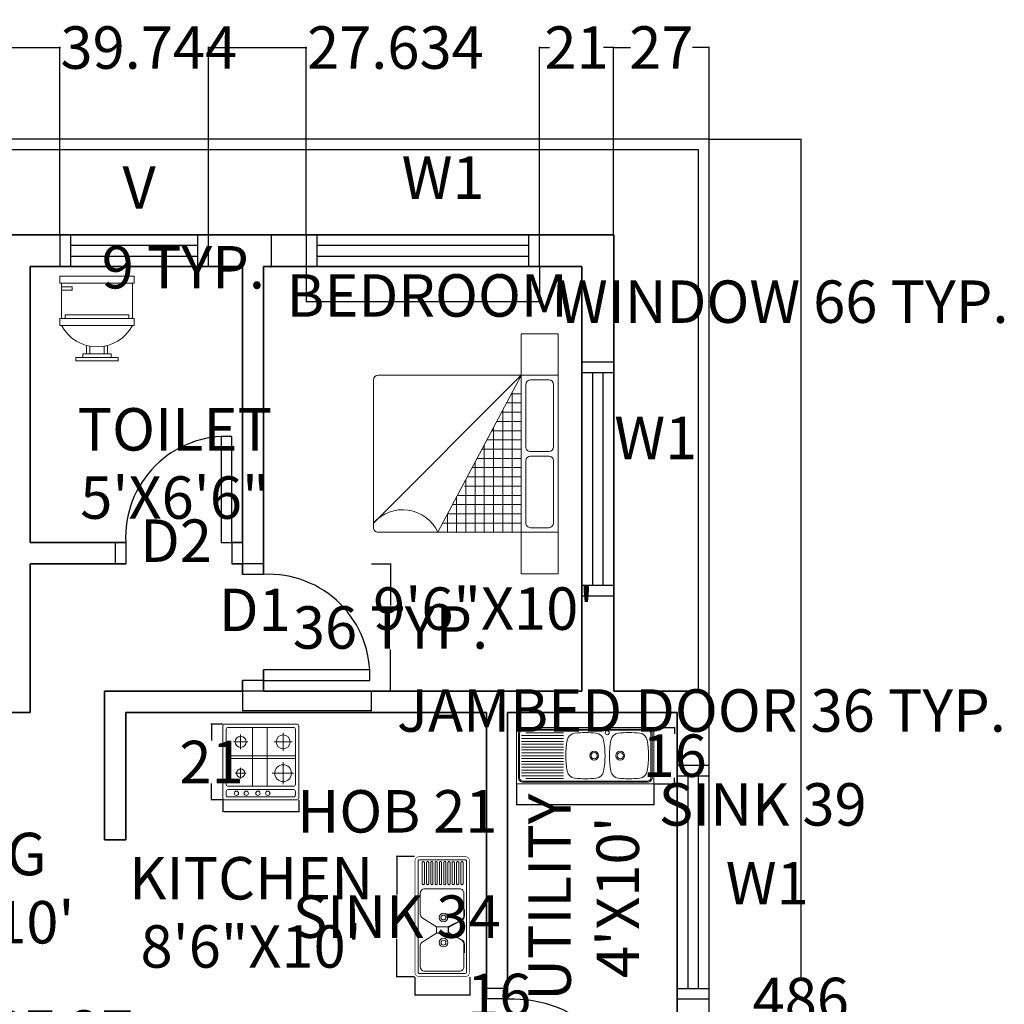
# Model space of a CAD drawing. Units: inches. Extents: x 774 to 1314, y 374 to 930.
# Tile 5 of 5: x 1035 to 1314, y 652 to 930. Entities that reach past the tile are written whole.
import ezdxf
from ezdxf.enums import TextEntityAlignment as Align

# ---------------------------------------------------------------- set-up
doc = ezdxf.new("R2010")
doc.units = ezdxf.units.IN
doc.header["$MEASUREMENT"] = 0
for name, color, linetype, lineweight in [('A-ANNO-DIMS', 2, 'Continuous', 18), ('A-ANNO-TEXT', 2, 'Continuous', 18), ('A-AREA-IDEN', 2, 'Continuous', 18), ('A-DOOR', 6, 'Continuous', 25), ('A-EQPM', 9, 'Continuous', 18), ('A-FLOR-FIXT', 9, 'Continuous', 18), ('A-FURN', 8, 'Continuous', 18), ('A-GLAZ', 4, 'Continuous', 18), ('A-WALL', 1, 'Continuous', 35), ('C-PROP', 3, 'Continuous', 25)]:
    doc.layers.add(name, color=color, linetype=linetype, lineweight=lineweight)
doc.layers.add('Layer4', color=4, linetype='Continuous')
doc.styles.get("Standard").update_dxf_attribs({"font": 'arial.ttf'})
doc.dimstyles.get("Standard").update_dxf_attribs({"dimtxt": 12, "dimasz": 0.18, "dimexe": 0.18, "dimexo": 0.0625, "dimgap": 0.09, "dimtad": 0, "dimtih": 1, "dimtoh": 1, "dimdec": 0, "dimzin": 0, "dimdsep": 46, "dimlunit": 4, "dimtxsty": 'Standard', "dimcen": 0.09, "dimadec": 0, "dimazin": 0, "dimtfac": 1, "dimtdec": 0, "dimtofl": 0, "dimtmove": 0, "dimatfit": 3, "dimfxl": 1, "dimtolj": 1, "dimtzin": 0, "dimarcsym": 0})

# ---------------------------------------------------------------- blocks, each defined once
blk = doc.blocks.new('ty')
at = {"layer": 'Layer4'}
for p, q in [((9, 42), (0, 42)), ((9, 39), (0, 39)), ((0, 39), (0, 3)), ((3, 39), (3, 3)), ((6, 3), (6, 39)), ((9, 3), (9, 39)), ((0, 3), (9, 3)), ((0, 0), (9, 0))]:
    blk.add_line(p, q, dxfattribs=at)
blk = doc.blocks.new('tr')
at = {"layer": 'Layer4'}
for p, q in [((9, 66), (0, 66)), ((9, 63), (0, 63)), ((0, 63), (0, 3)), ((3, 63), (3, 3)), ((6, 3), (6, 63)), ((9, 3), (9, 63)), ((0, 3), (9, 3)), ((0, 0), (9, 0))]:
    blk.add_line(p, q, dxfattribs=at)
blk = doc.blocks.new('A$C4CBC1980')
for p, q in [((0.45, 2), (0, 2)), ((0, 2), (0, 1.6)), ((0, 2), (2.6, 2)), ((2.15, 2), (0.45, 2)), ((0.45, 2), (0.45, 0.05)), ((0.45, 0.05), (0.45, 2)), ((1.225, 1.95), (0.55, 1.95)), ((2.05, 1.95), (1.375, 1.95)), ((2.6, 2), (2.025, 2)), ((2.15, 0.05), (2.15, 2)), ((2.6, 1.6), (2.6, 2)), ((0.5, 1.9), (0.5, 1.7)), ((1.275, 1.7), (1.275, 1.9)), ((1.325, 1.7), (1.325, 1.9)), ((2.1, 1.7), (2.1, 1.9)), ((2.6, 1.6), (0, 1.6)), ((0.45, 1.6), (2.05, 0)), ((0.451, 1.6), (2.15, 0.697)), ((1.225, 1.65), (0.55, 1.65)), ((2.15, 1.6), (0.587, 1.6)), ((0.65, 1.494), (0.65, 1.6)), ((0.75, 1.441), (0.75, 1.6)), ((0.85, 1.388), (0.85, 1.6)), ((0.95, 1.335), (0.95, 1.6)), ((1.05, 1.282), (1.05, 1.6)), ((1.15, 1.229), (1.15, 1.6)), ((1.25, 1.176), (1.25, 1.6)), ((1.35, 1.122), (1.35, 1.6)), ((2.05, 1.65), (1.375, 1.65)), ((1.45, 1.069), (1.45, 1.6)), ((1.55, 1.016), (1.55, 1.6)), ((1.65, 0.986), (1.65, 1.6)), ((1.75, 0.91), (1.75, 1.6)), ((1.85, 0.857), (1.85, 1.6)), ((1.95, 0.804), (1.95, 1.6)), ((2.05, 0.751), (2.05, 1.6)), ((2.15, 1.5), (0.639, 1.5)), ((2.15, 1.4), (0.827, 1.4)), ((2.15, 1.3), (1.016, 1.3)), ((2.15, 1.2), (1.204, 1.2)), ((2.15, 1.1), (1.392, 1.1)), ((2.15, 1), (1.58, 1)), ((2.15, 0.9), (1.769, 0.9)), ((2.15, 0.8), (1.957, 0.8)), ((0.5, 0), (2.1, 0))]:
    blk.add_line(p, q)
for centre, radius, start, end in [((0.55, 1.9), 0.05, 90, 180), ((1.225, 1.9), 0.05, 0, 90), ((1.375, 1.9), 0.05, 90, 180), ((2.05, 1.9), 0.05, 0, 90), ((0.55, 1.7), 0.05, 180, 270), ((1.225, 1.7), 0.05, 270, 0), ((1.375, 1.7), 0.05, 180, 270), ((2.05, 1.7), 0.05, 270, 0), ((2.327, 0.316), 0.421, 114.9633, 228.7161), ((0.5, 0.05), 0.05, 180, 270), ((0.5, 0.05), 0.05, 180, 270), ((2.1, 0.05), 0.05, 270, 0)]:
    blk.add_arc(centre, radius, start, end)
blk = doc.blocks.new('A$C44FE756A')
for p, q in [((57.4, 450.3), (254.8, 450.3)), ((57.4, 430.3), (254.8, 430.3)), ((57.4, 410.3), (254.8, 410.3)), ((57.4, 390.3), (254.8, 390.3)), ((57.4, 370.3), (254.8, 370.3)), ((57.4, 350.3), (254.8, 350.3)), ((57.4, 330.3), (254.8, 330.3)), ((57.4, 310.3), (254.8, 310.3)), ((57.4, 290.3), (254.8, 290.3)), ((659.7, 311.5), (711.5, 311.5)), ((57.4, 270.3), (254.8, 270.3)), ((57.4, 250.3), (254.8, 250.3)), ((57.4, 230.3), (254.8, 230.3)), ((57.4, 210.3), (254.8, 210.3)), ((57.4, 190.3), (254.8, 190.3)), ((658.1, 202.9), (709.9, 202.9)), ((57.4, 170.3), (254.8, 170.3)), ((57.4, 150.3), (254.8, 150.3)), ((57.4, 130.3), (254.8, 130.3)), ((57.4, 110.3), (254.8, 110.3)), ((57.4, 90.3), (254.8, 90.3)), ((57.4, 70.3), (254.8, 70.3))]:
    blk.add_line(p, q)
at = {"const_width": 5}
blk.add_lwpolyline([(296.3, 511.5), (42.5, 511.5, 0.414214), (2.5, 471.5), (2.5, 42.5, 0.414214), (42.5, 2.5), (296.3, 2.5), (1080.4, 2.5, 0.414214), (1120.4, 42.5), (1120.4, 471.5, 0.414214), (1080.4, 511.5)], format="xyb", close=True, dxfattribs=at)
for points in [[(296.3, 32.5), (42.5, 32.5, -0.414214), (32.5, 42.5), (32.5, 471.5, -0.414214), (42.5, 481.5), (296.3, 481.5), (1080.4, 481.5, -0.414214), (1090.4, 471.5), (1090.4, 42.5, -0.414214), (1080.4, 32.5), (296.2, 32.5)], [(496.2, 464), (554.7, 464, -0.277085), (594.4, 440.1), (658.1, 320.7, 0.277085), (665.1, 316.5), (706.1, 316.5, 0.277085), (713.2, 320.7), (776.8, 440.1, -0.277085), (816.5, 464), (899.4, 464)]]:
    blk.add_lwpolyline(points, format="xyb")
for points in [[(651.8, 321.9, -0.123011), (656.5, 303.1), (656.5, 204.5), (572.7, 70.9, -0.258191), (538.8, 52.2), (341.8, 52.2, -0.414214), (301.8, 92.2), (301.8, 419, -0.414214), (341.8, 459), (554.7, 459, -0.277085), (590, 437.8)], [(816.5, 459, 0.277085), (781.2, 437.8), (719.5, 321.9, 0.123011), (714.8, 303.1), (714.8, 204.5), (798.5, 70.9, 0.258191), (832.4, 52.2), (1029.4, 52.2, 0.414214), (1069.4, 92.2), (1069.4, 419, 0.414214), (1029.4, 459)]]:
    blk.add_lwpolyline(points, format="xyb", close=True)
for centre, radius in [((569, 267.7), 40.5), ((569, 267.7), 22.7), ((803.8, 267.7), 40.5), ((803.8, 267.7), 22.7)]:
    blk.add_circle(centre, radius)
for centre, start, end in [((57.4, 440.3), 89.99997, 270.00003), ((57.4, 400.3), 89.99997, 270.00003), ((57.4, 360.3), 89.99997, 270.00003), ((254.8, 440.3), 268.86024, 91.13976), ((254.8, 400.3), 268.86024, 91.13976), ((254.8, 360.3), 268.86024, 91.13976), ((57.4, 320.3), 89.99997, 270.00003), ((57.4, 280.3), 89.99997, 270.00003), ((254.8, 320.3), 268.86024, 91.13976), ((254.8, 280.3), 268.86024, 91.13976), ((57.4, 240.3), 89.99997, 270.00003), ((57.4, 200.3), 89.99997, 270.00003), ((254.8, 240.3), 268.86024, 91.13976), ((254.8, 200.3), 268.86024, 91.13976), ((57.4, 160.3), 89.99997, 270.00003), ((57.4, 120.3), 89.99997, 270.00003), ((254.8, 160.3), 268.86024, 91.13976), ((254.8, 120.3), 268.86024, 91.13976), ((57.4, 80.3), 89.99997, 270.00003), ((254.8, 80.3), 268.86024, 91.13976)]:
    blk.add_arc(centre, 10, start, end)
blk = doc.blocks.new('A$C04B7649A')
for p, q in [((462.1, 500.4), (90.9, 500.4)), ((462.1, 472.3), (50.6, 472.3)), ((462.1, 444.1), (50.6, 444.1)), ((462.1, 416), (50.6, 416)), ((462.1, 387.9), (50.6, 387.9)), ((462.1, 359.8), (50.6, 359.8)), ((462.1, 331.7), (50.6, 331.7)), ((462.1, 303.6), (50.6, 303.6)), ((1319.5, 275.5), (1319.5, 308.5)), ((462.1, 275.5), (50.6, 275.5)), ((462.1, 247.4), (50.6, 247.4)), ((462.1, 219.3), (50.6, 219.3)), ((462.1, 191.2), (50.6, 191.2)), ((462.1, 163), (50.6, 163)), ((462.1, 134.9), (50.6, 134.9)), ((462.1, 106.8), (50.6, 106.8)), ((462.1, 78.7), (50.6, 78.7)), ((462.1, 50.6), (93.2, 50.6))]:
    blk.add_line(p, q)
blk.add_lwpolyline([(0, 0), (1349.3, 0), (1349.3, 551), (0, 551)], close=True)
for points in [[(18.6, 491.9), (18.6, 59, 0.414214), (63.5, 14.1), (1285.8, 14.1, 0.414214), (1330.8, 59), (1330.8, 491.9, 0.414214), (1285.8, 536.9), (63.5, 536.9, 0.414214)], [(29.8, 491.9), (29.8, 59, 0.414214), (63.5, 25.3), (1285.8, 25.3, 0.414214), (1319.5, 59), (1319.5, 491.9, 0.414214), (1285.8, 525.7), (63.5, 525.7, 0.414214)], [(570.8, 495.9, 0.326796), (498.4, 427.4, 0.090842), (498.4, 123.5, 0.326796), (570.8, 55.1, 0.063178), (783, 55.1, 0.326796), (855.4, 123.5, 0.090842), (855.4, 427.4, 0.326796), (783, 495.9, 0.063178)], [(998, 495.9, 0.326796), (925.7, 427.4, 0.090842), (925.7, 123.5, 0.326796), (998, 55.1, 0.063178), (1210.3, 55.1, 0.326796), (1282.7, 123.5, 0.090842), (1282.7, 427.4, 0.326796), (1210.3, 495.9, 0.063178)]]:
    blk.add_lwpolyline(points, format="xyb", close=True)
for centre, radius in [((890.5, 500.4), 19.7), ((762.4, 275.5), 42.7), ((762.4, 275.5), 30.9), ((1018.7, 275.5), 42.7), ((1018.7, 275.5), 30.9)]:
    blk.add_circle(centre, radius)
blk = doc.blocks.new('23')
at = {"color": 0}
for p, q in [((4420.74, 13532.6), (4420.74, 13584.6)), ((4422.24, 13586.1), (4474.24, 13586.1)), ((4424.64, 13583.7), (4464.32, 13583.7)), ((4443.77, 13583.7), (4443.77, 13533.5)), ((4445.71, 13583.7), (4445.71, 13533.5)), ((4456.31, 13582.63), (4456.31, 13566.88)), ((4469.72, 13583.68), (4472.04, 13583.68)), ((4475.74, 13584.6), (4475.74, 13532.6)), ((4423.14, 13535), (4423.14, 13582.2)), ((4433.62, 13581.32), (4433.62, 13568.19)), ((4465.82, 13582.2), (4465.82, 13535)), ((4468.22, 13582.18), (4468.22, 13534.86)), ((4468.22, 13582.18), (4468.22, 13534.86)), ((4473.54, 13582.18), (4473.54, 13534.86)), ((4427.06, 13574.75), (4440.18, 13574.75)), ((4448.43, 13574.75), (4464.18, 13574.75)), ((4423.14, 13563.17), (4465.82, 13563.17)), ((4423.14, 13552.44), (4465.82, 13552.44)), ((4433.62, 13549.21), (4433.62, 13538.71)), ((4456.31, 13547.9), (4456.31, 13540.03)), ((4428.37, 13543.96), (4438.87, 13543.96)), ((4452.37, 13543.96), (4460.24, 13543.96)), ((4464.32, 13533.5), (4424.64, 13533.5)), ((4472.04, 13533.36), (4469.72, 13533.36)), ((4474.24, 13531.1), (4422.24, 13531.1))]:
    blk.add_line(p, q, dxfattribs=at)
for centre, radius in [((4433.62, 13574.75), 5.04), ((4456.31, 13574.75), 6.05), ((4470.88, 13563.64), 1.57), ((4470.88, 13556.51), 1.57), ((4433.62, 13543.96), 4.03), ((4456.31, 13543.96), 3.03), ((4470.88, 13548.02), 1.57), ((4470.88, 13540.9), 1.57)]:
    blk.add_circle(centre, radius, dxfattribs=at)
for centre, start, end in [((4422.24, 13584.6), 90, 180), ((4424.64, 13582.2), 90, 180), ((4464.32, 13582.2), 0, 90), ((4469.72, 13582.18), 90, 180), ((4472.04, 13582.18), 0, 90), ((4474.24, 13584.6), 0, 90), ((4424.64, 13535), 180, 270), ((4464.32, 13535), 270, 0), ((4469.72, 13534.86), 180, 270), ((4472.04, 13534.86), 270, 0), ((4422.24, 13532.6), 180, 270), ((4474.24, 13532.6), 270, 0)]:
    blk.add_arc(centre, 1.5, start, end, dxfattribs=at)
blk = doc.blocks.new('*U18')
for p, q in [((-10, 22), (-10, 12)), ((-10, 21), (-7, 21)), ((-7, 20), (-10, 20)), ((-7, 21), (-7, 20)), ((10, 12), (10, 22)), ((10.5, 12), (-10.5, 12)), ((-10.5, 10), (-10.5, 12)), ((9, 13), (-9, 13)), ((-9, 13), (-9, 12)), ((9, 12), (9, 13)), ((10.5, 12), (10.5, 10)), ((10.5, 10), (-10.5, 10)), ((-3, 4.4065), (-3, 2)), ((-2, 2), (-2, 4.1658)), ((2, 4.1658), (2, 2)), ((3, 2), (3, 4.4065)), ((4, 2), (-4, 2)), ((-4, 2), (-4, 1)), ((4, 1), (4, 2))]:
    blk.add_line(p, q)
for points in [[(10.5, 22), (10.5, 24), (-10.5, 24), (-10.5, 22)], [(6, 0), (6, 1), (-6, 1), (-6, 0)]]:
    blk.add_lwpolyline(points, close=True)
blk.add_arc((0, 15.3333), 11.3333, 208.0725, 331.9275)
blk = doc.blocks.new('DOOR-SWING-36IN')
blk.add_lwpolyline([(0, 0), (3, 0), (3, 36), (0, 36)], close=True)
blk.add_arc((1.5, 1.5), 34.53, 357.5104, 92.4896)
blk = doc.blocks.new('DOOR-30IN-6IN-JAMB')
for p, q in [((6, 36), (0, 36)), ((6, 33), (0, 33)), ((6, 3), (0, 3)), ((6, 0), (0, 0))]:
    blk.add_line(p, q)
blk.add_lwpolyline([(6, 3), (36, 3), (36, 6), (6, 6)], close=True)
blk.add_arc((7.5, 4.5), 28.54, 356.9872, 93.0128)
blk = doc.blocks.new('*D25')
at = {"layer": 'A-ANNO-DIMS', "color": 0, "lineweight": -2, "transparency": 16777216}
for p, q in [((1116.33, 860.5), (1116.33, 850.49)), ((1182.33, 860.5), (1182.33, 850.49)), ((1116.51, 850.67), (1182.15, 850.67)), ((1182.33, 850.67), (1182.51, 850.67))]:
    blk.add_line(p, q, dxfattribs=at)
at = {"layer": 'A-ANNO-DIMS', "color": 0, "transparency": 16777216}
for points in [[(1116.51, 850.7), (1116.51, 850.64), (1116.33, 850.67)], [(1182.15, 850.7), (1182.15, 850.64), (1182.33, 850.67)]]:
    blk.add_solid(points, dxfattribs=at)
at = {"layer": 'Defpoints', "color": 0, "transparency": 16777216}
for p in [(1116.33, 860.57), (1182.33, 860.57), (1182.33, 850.67)]:
    blk.add_point(p, dxfattribs=at)
at = {"layer": 'A-ANNO-DIMS', "color": 0, "transparency": 16777216, "insert": (1251.16, 850.67), "char_height": 12, "attachment_point": 5}
blk.add_mtext('\\A1;WINDOW 66 TYP.', dxfattribs=at)
blk = doc.blocks.new('*D26')
at = {"layer": 'A-ANNO-DIMS', "color": 0, "lineweight": -2, "transparency": 16777216}
for p, q in [((1116.27, 869.57), (1106.25, 869.57)), ((1106.43, 869.39), (1106.43, 860.75)), ((1116.27, 860.57), (1106.25, 860.57)), ((1106.43, 860.57), (1106.43, 860.39)), ((1106.43, 860.39), (1106.25, 860.39))]:
    blk.add_line(p, q, dxfattribs=at)
at = {"layer": 'A-ANNO-DIMS', "color": 0, "transparency": 16777216}
for points in [[(1106.4, 869.39), (1106.46, 869.39), (1106.43, 869.57)], [(1106.4, 860.75), (1106.46, 860.75), (1106.43, 860.57)]]:
    blk.add_solid(points, dxfattribs=at)
at = {"layer": 'Defpoints', "color": 0, "transparency": 16777216}
for p in [(1116.33, 869.57), (1106.43, 860.57), (1116.33, 860.57)]:
    blk.add_point(p, dxfattribs=at)
at = {"layer": 'A-ANNO-DIMS', "color": 0, "transparency": 16777216, "insert": (1081.62, 860.39), "char_height": 12, "attachment_point": 5}
blk.add_mtext('\\A1;9 TYP.', dxfattribs=at)
blk = doc.blocks.new('*D31')
at = {"layer": 'A-ANNO-DIMS', "color": 0, "lineweight": -2, "transparency": 16777216}
for p, q in [((1098.33, 740.5), (1098.33, 734.92)), ((1134.76, 740.5), (1134.76, 734.92)), ((1098.51, 735.1), (1134.58, 735.1)), ((1134.76, 735.1), (1134.94, 735.1))]:
    blk.add_line(p, q, dxfattribs=at)
at = {"layer": 'A-ANNO-DIMS', "color": 0, "transparency": 16777216}
for points in [[(1098.51, 735.13), (1098.51, 735.07), (1098.33, 735.1)], [(1134.58, 735.13), (1134.58, 735.07), (1134.76, 735.1)]]:
    blk.add_solid(points, dxfattribs=at)
at = {"layer": 'Defpoints', "color": 0, "transparency": 16777216}
for p in [(1098.33, 740.57), (1134.76, 740.57), (1134.76, 735.1)]:
    blk.add_point(p, dxfattribs=at)
at = {"layer": 'A-ANNO-DIMS', "color": 0, "transparency": 16777216, "insert": (1228.16, 735.1), "char_height": 12, "attachment_point": 5}
blk.add_mtext('\\A1;JAMBED DOOR 36 TYP.', dxfattribs=at)
blk = doc.blocks.new('*D32')
at = {"layer": 'A-ANNO-DIMS', "color": 0, "lineweight": -2, "transparency": 16777216}
for p, q in [((1134.82, 776.57), (1140.4, 776.57)), ((1140.22, 776.39), (1140.22, 764.79)), ((1140.22, 740.75), (1140.22, 752.34)), ((1134.82, 740.57), (1140.4, 740.57))]:
    blk.add_line(p, q, dxfattribs=at)
at = {"layer": 'A-ANNO-DIMS', "color": 0, "transparency": 16777216}
for points in [[(1140.19, 776.39), (1140.25, 776.39), (1140.22, 776.57)], [(1140.19, 740.75), (1140.25, 740.75), (1140.22, 740.57)]]:
    blk.add_solid(points, dxfattribs=at)
at = {"layer": 'Defpoints', "color": 0, "transparency": 16777216}
for p in [(1134.76, 776.57), (1140.22, 776.57), (1134.76, 740.57)]:
    blk.add_point(p, dxfattribs=at)
at = {"layer": 'A-ANNO-DIMS', "color": 0, "transparency": 16777216, "insert": (1140.22, 758.57), "char_height": 12, "attachment_point": 5}
blk.add_mtext('\\A1;36 TYP.', dxfattribs=at)
blk = doc.blocks.new('*D45')
at = {"layer": 'A-ANNO-DIMS', "color": 0, "lineweight": -2, "transparency": 16777216}
for p, q in [((1147, 693.87), (1141.78, 693.87)), ((1141.96, 693.69), (1141.96, 683.14)), ((1141.96, 660), (1141.96, 670.54)), ((1147, 659.82), (1141.78, 659.82))]:
    blk.add_line(p, q, dxfattribs=at)
at = {"layer": 'A-ANNO-DIMS', "color": 0, "transparency": 16777216}
for points in [[(1141.93, 693.69), (1141.99, 693.69), (1141.96, 693.87)], [(1141.93, 660), (1141.99, 660), (1141.96, 659.82)]]:
    blk.add_solid(points, dxfattribs=at)
at = {"layer": 'Defpoints', "color": 0, "transparency": 16777216}
for p in [(1147.06, 693.87), (1141.96, 659.82), (1147.06, 659.82)]:
    blk.add_point(p, dxfattribs=at)
at = {"layer": 'A-ANNO-DIMS', "color": 0, "transparency": 16777216, "insert": (1141.96, 676.84), "char_height": 12, "attachment_point": 5}
blk.add_mtext('\\A1;SINK 34', dxfattribs=at)
blk = doc.blocks.new('*D46')
at = {"layer": 'A-ANNO-DIMS', "color": 0, "lineweight": -2, "transparency": 16777216}
for p, q in [((1147.06, 659.75), (1147.06, 654.53)), ((1162.65, 659.75), (1162.65, 654.53)), ((1147.24, 654.71), (1162.47, 654.71)), ((1162.65, 654.71), (1162.83, 654.71))]:
    blk.add_line(p, q, dxfattribs=at)
at = {"layer": 'A-ANNO-DIMS', "color": 0, "transparency": 16777216}
for points in [[(1147.24, 654.74), (1147.24, 654.68), (1147.06, 654.71)], [(1162.47, 654.74), (1162.47, 654.68), (1162.65, 654.71)]]:
    blk.add_solid(points, dxfattribs=at)
at = {"layer": 'Defpoints', "color": 0, "transparency": 16777216}
for p in [(1147.06, 659.82), (1162.65, 659.82), (1162.65, 654.71)]:
    blk.add_point(p, dxfattribs=at)
at = {"layer": 'A-ANNO-DIMS', "color": 0, "transparency": 16777216, "insert": (1170.95, 654.71), "char_height": 12, "attachment_point": 5}
blk.add_mtext('\\A1;16', dxfattribs=at)
blk = doc.blocks.new('*D47')
at = {"layer": 'A-ANNO-DIMS', "color": 0, "lineweight": -2, "transparency": 16777216}
for p, q in [((1175.84, 714.34), (1175.84, 708.38)), ((1214.74, 714.34), (1214.74, 708.38)), ((1176.02, 708.56), (1214.56, 708.56)), ((1214.74, 708.56), (1214.92, 708.56))]:
    blk.add_line(p, q, dxfattribs=at)
at = {"layer": 'A-ANNO-DIMS', "color": 0, "transparency": 16777216}
for points in [[(1176.02, 708.59), (1176.02, 708.53), (1175.84, 708.56)], [(1214.56, 708.59), (1214.56, 708.53), (1214.74, 708.56)]]:
    blk.add_solid(points, dxfattribs=at)
at = {"layer": 'Defpoints', "color": 0, "transparency": 16777216}
for p in [(1175.84, 714.4), (1214.74, 714.4), (1214.74, 708.56)]:
    blk.add_point(p, dxfattribs=at)
at = {"layer": 'A-ANNO-DIMS', "color": 0, "transparency": 16777216, "insert": (1245.48, 708.56), "char_height": 12, "attachment_point": 5}
blk.add_mtext('\\A1;SINK 39', dxfattribs=at)
blk = doc.blocks.new('*D48')
at = {"layer": 'A-ANNO-DIMS', "color": 0, "lineweight": -2, "transparency": 16777216}
for p, q in [((1214.8, 730.28), (1220.75, 730.28)), ((1220.57, 730.1), (1220.57, 728.56)), ((1220.57, 714.58), (1220.57, 716.12)), ((1214.8, 714.4), (1220.75, 714.4))]:
    blk.add_line(p, q, dxfattribs=at)
at = {"layer": 'A-ANNO-DIMS', "color": 0, "transparency": 16777216}
for points in [[(1220.54, 730.1), (1220.6, 730.1), (1220.57, 730.28)], [(1220.54, 714.58), (1220.6, 714.58), (1220.57, 714.4)]]:
    blk.add_solid(points, dxfattribs=at)
at = {"layer": 'Defpoints', "color": 0, "transparency": 16777216}
for p in [(1214.74, 730.28), (1220.57, 730.28), (1214.74, 714.4)]:
    blk.add_point(p, dxfattribs=at)
at = {"layer": 'A-ANNO-DIMS', "color": 0, "transparency": 16777216, "insert": (1220.57, 722.34), "char_height": 12, "attachment_point": 5}
blk.add_mtext('\\A1;16', dxfattribs=at)
blk = doc.blocks.new('*D49')
at = {"layer": 'A-ANNO-DIMS', "color": 0, "lineweight": -2, "transparency": 16777216}
for p, q in [((1092.81, 709.76), (1092.81, 706.42)), ((1114.27, 709.76), (1114.27, 706.42)), ((1092.99, 706.6), (1114.09, 706.6)), ((1114.27, 706.6), (1114.45, 706.6))]:
    blk.add_line(p, q, dxfattribs=at)
at = {"layer": 'A-ANNO-DIMS', "color": 0, "transparency": 16777216}
for points in [[(1092.99, 706.63), (1092.99, 706.57), (1092.81, 706.6)], [(1114.09, 706.63), (1114.09, 706.57), (1114.27, 706.6)]]:
    blk.add_solid(points, dxfattribs=at)
at = {"layer": 'Defpoints', "color": 0, "transparency": 16777216}
for p in [(1092.81, 709.82), (1114.27, 709.82), (1114.27, 706.6)]:
    blk.add_point(p, dxfattribs=at)
at = {"layer": 'A-ANNO-DIMS', "color": 0, "transparency": 16777216, "insert": (1142.15, 706.6), "char_height": 12, "attachment_point": 5}
blk.add_mtext('\\A1;HOB 21', dxfattribs=at)
blk = doc.blocks.new('*D50')
at = {"layer": 'A-ANNO-DIMS', "color": 0, "lineweight": -2, "transparency": 16777216}
for p, q in [((1092.75, 731.28), (1089.41, 731.28)), ((1089.59, 731.1), (1089.59, 726.66)), ((1089.59, 710), (1089.59, 714.43)), ((1092.75, 709.82), (1089.41, 709.82))]:
    blk.add_line(p, q, dxfattribs=at)
at = {"layer": 'A-ANNO-DIMS', "color": 0, "transparency": 16777216}
for points in [[(1089.56, 731.1), (1089.62, 731.1), (1089.59, 731.28)], [(1089.56, 710), (1089.62, 710), (1089.59, 709.82)]]:
    blk.add_solid(points, dxfattribs=at)
at = {"layer": 'Defpoints', "color": 0, "transparency": 16777216}
for p in [(1092.81, 731.28), (1089.59, 709.82), (1092.81, 709.82)]:
    blk.add_point(p, dxfattribs=at)
at = {"layer": 'A-ANNO-DIMS', "color": 0, "transparency": 16777216, "insert": (1089.59, 720.55), "char_height": 12, "attachment_point": 5}
blk.add_mtext('\\A1;21', dxfattribs=at)
blk = doc.blocks.new('*D51')
at = {"layer": 'A-ANNO-DIMS', "color": 0, "lineweight": -2, "transparency": 16777216}
for p, q in [((1072.03, 644.35), (1071.85, 644.35)), ((1072.03, 640.32), (1072.03, 644.53)), ((1099.12, 644.35), (1072.21, 644.35)), ((1099.3, 640.32), (1099.3, 644.53))]:
    blk.add_line(p, q, dxfattribs=at)
at = {"layer": 'A-ANNO-DIMS', "color": 0, "transparency": 16777216}
for points in [[(1072.21, 644.38), (1072.21, 644.32), (1072.03, 644.35)], [(1099.12, 644.38), (1099.12, 644.32), (1099.3, 644.35)]]:
    blk.add_solid(points, dxfattribs=at)
at = {"layer": 'Defpoints', "color": 0, "transparency": 16777216}
for p in [(1072.03, 644.35), (1072.03, 640.25), (1099.3, 640.25)]:
    blk.add_point(p, dxfattribs=at)
at = {"layer": 'A-ANNO-DIMS', "color": 0, "transparency": 16777216, "insert": (1013.43, 644.35), "char_height": 12, "attachment_point": 5}
blk.add_mtext('\\A1;APPLIANCE 27', dxfattribs=at)
blk = doc.blocks.new('*D54')
at = {"layer": 'A-ANNO-DIMS', "color": 0, "lineweight": -2, "transparency": 16777216}
for p, q in [((1230.4, 896.57), (1256.44, 896.57)), ((1256.26, 896.39), (1256.26, 659.78)), ((1256.26, 410.75), (1256.26, 647.35)), ((1230.4, 410.57), (1256.44, 410.57))]:
    blk.add_line(p, q, dxfattribs=at)
at = {"layer": 'A-ANNO-DIMS', "color": 0, "transparency": 16777216}
for points in [[(1256.23, 896.39), (1256.29, 896.39), (1256.26, 896.57)], [(1256.23, 410.75), (1256.29, 410.75), (1256.26, 410.57)]]:
    blk.add_solid(points, dxfattribs=at)
at = {"layer": 'Defpoints', "color": 0, "transparency": 16777216}
for p in [(1230.33, 896.57), (1256.26, 896.57), (1230.33, 410.57)]:
    blk.add_point(p, dxfattribs=at)
at = {"layer": 'A-ANNO-DIMS', "color": 0, "transparency": 16777216, "insert": (1256.26, 653.57), "char_height": 12, "attachment_point": 5}
blk.add_mtext('\\A1;486', dxfattribs=at)
blk = doc.blocks.new('*D57')
at = {"layer": 'A-ANNO-DIMS', "color": 0, "lineweight": -2, "transparency": 16777216}
for p, q in [((1006.96, 869.63), (1006.96, 922.67)), ((1007.14, 922.49), (1046.52, 922.49)), ((1046.7, 869.63), (1046.7, 922.67)), ((1046.7, 922.49), (1046.88, 922.49))]:
    blk.add_line(p, q, dxfattribs=at)
at = {"layer": 'A-ANNO-DIMS', "color": 0, "transparency": 16777216}
for points in [[(1007.14, 922.52), (1007.14, 922.46), (1006.96, 922.49)], [(1046.52, 922.52), (1046.52, 922.46), (1046.7, 922.49)]]:
    blk.add_solid(points, dxfattribs=at)
at = {"layer": 'Defpoints', "color": 0, "transparency": 16777216}
for p in [(1046.7, 922.49), (1006.96, 869.57), (1046.7, 869.57)]:
    blk.add_point(p, dxfattribs=at)
at = {"layer": 'A-ANNO-DIMS', "color": 0, "transparency": 16777216, "insert": (1071.85, 922.49), "char_height": 12, "attachment_point": 5}
blk.add_mtext('\\A1;39.744', dxfattribs=at)
blk = doc.blocks.new('*D58')
at = {"layer": 'A-ANNO-DIMS', "color": 0, "lineweight": -2, "transparency": 16777216}
for p, q in [((1088.7, 869.63), (1088.7, 922.67)), ((1088.88, 922.49), (1116.15, 922.49)), ((1116.33, 869.63), (1116.33, 922.67)), ((1116.33, 922.49), (1116.51, 922.49))]:
    blk.add_line(p, q, dxfattribs=at)
at = {"layer": 'A-ANNO-DIMS', "color": 0, "transparency": 16777216}
for points in [[(1088.88, 922.52), (1088.88, 922.46), (1088.7, 922.49)], [(1116.15, 922.52), (1116.15, 922.46), (1116.33, 922.49)]]:
    blk.add_solid(points, dxfattribs=at)
at = {"layer": 'Defpoints', "color": 0, "transparency": 16777216}
for p in [(1116.33, 922.49), (1088.7, 869.57), (1116.33, 869.57)]:
    blk.add_point(p, dxfattribs=at)
at = {"layer": 'A-ANNO-DIMS', "color": 0, "transparency": 16777216, "insert": (1141.59, 922.49), "char_height": 12, "attachment_point": 5}
blk.add_mtext('\\A1;27.634', dxfattribs=at)
blk = doc.blocks.new('*D59')
at = {"layer": 'A-ANNO-DIMS', "color": 0, "lineweight": -2, "transparency": 16777216}
for p, q in [((1182.33, 869.63), (1182.33, 922.67)), ((1182.51, 922.49), (1185.21, 922.49)), ((1203.15, 922.49), (1200.46, 922.49)), ((1203.33, 869.63), (1203.33, 922.67))]:
    blk.add_line(p, q, dxfattribs=at)
at = {"layer": 'A-ANNO-DIMS', "color": 0, "transparency": 16777216}
for points in [[(1182.51, 922.52), (1182.51, 922.46), (1182.33, 922.49)], [(1203.15, 922.52), (1203.15, 922.46), (1203.33, 922.49)]]:
    blk.add_solid(points, dxfattribs=at)
at = {"layer": 'Defpoints', "color": 0, "transparency": 16777216}
for p in [(1203.33, 922.49), (1182.33, 869.57), (1203.33, 869.57)]:
    blk.add_point(p, dxfattribs=at)
at = {"layer": 'A-ANNO-DIMS', "color": 0, "transparency": 16777216, "insert": (1192.83, 922.49), "char_height": 12, "attachment_point": 5}
blk.add_mtext('\\A1;21', dxfattribs=at)
blk = doc.blocks.new('*D60')
at = {"layer": 'A-ANNO-DIMS', "color": 0, "lineweight": -2, "transparency": 16777216}
for p, q in [((1203.33, 869.63), (1203.33, 922.67)), ((1203.51, 922.49), (1208.05, 922.49)), ((1230.15, 922.49), (1225.62, 922.49)), ((1230.33, 896.63), (1230.33, 922.67))]:
    blk.add_line(p, q, dxfattribs=at)
at = {"layer": 'A-ANNO-DIMS', "color": 0, "transparency": 16777216}
for points in [[(1203.51, 922.52), (1203.51, 922.46), (1203.33, 922.49)], [(1230.15, 922.52), (1230.15, 922.46), (1230.33, 922.49)]]:
    blk.add_solid(points, dxfattribs=at)
at = {"layer": 'Defpoints', "color": 0, "transparency": 16777216}
for p in [(1230.33, 922.49), (1230.33, 896.57), (1203.33, 869.57)]:
    blk.add_point(p, dxfattribs=at)
at = {"layer": 'A-ANNO-DIMS', "color": 0, "transparency": 16777216, "insert": (1216.83, 922.49), "char_height": 12, "attachment_point": 5}
blk.add_mtext('\\A1;27', dxfattribs=at)

msp = doc.modelspace()

# ---------------------------------------------------------------- linework, layer by layer
at = {"layer": 'A-DOOR'}
for p, q in [((1173.3347, 656.5656), (1167.3347, 656.5656)), ((1173.3347, 653.5656), (1167.3347, 653.5656))]:
    msp.add_line(p, q, dxfattribs=at)
at = {"layer": 'A-WALL'}
for p, q in [((1038.3347, 860.5656), (1038.3347, 782.5656)), ((1098.3347, 860.5656), (1038.3347, 860.5656)), ((1098.3347, 860.5656), (1098.3347, 782.5656)), ((1194.3347, 860.5656), (1104.3347, 860.5656)), ((1104.3347, 860.5656), (1104.3347, 773.5656)), ((1194.3347, 740.5656), (1194.3347, 860.5656)), ((1065.3347, 782.5656), (1038.3347, 782.5656)), ((1098.3347, 782.5656), (1095.3347, 782.5656)), ((1038.3347, 776.5656), (1038.3347, 734.5656)), ((1065.3347, 776.5656), (1038.3347, 776.5656)), ((1098.3347, 776.5656), (1095.3347, 776.5656)), ((1098.3347, 776.5656), (1098.3347, 773.5656)), ((1104.3347, 746.5656), (1104.3347, 740.5656)), ((1098.3347, 743.5656), (1098.3347, 740.5656)), ((1098.3347, 740.5656), (1059.3347, 740.5656)), ((1194.3347, 740.5656), (1104.3347, 740.5656)), ((1227.3347, 740.5656), (1203.3347, 740.5656)), ((1038.3347, 734.5656), (1029.3347, 734.5656)), ((1140.3347, 734.5656), (1065.3347, 734.5656)), ((1167.3347, 734.5656), (1065.3347, 734.5656)), ((1221.3347, 734.5656), (1173.3347, 734.5656)), ((1065.3347, 698.5656), (1059.3347, 698.5656))]:
    msp.add_line(p, q, dxfattribs=at)
for points in [[(1203.3347, 740.5656), (1203.3347, 869.5656), (891.3347, 869.5656), (891.3347, 527.5656)], [(1059.3347, 698.5656), (1059.3347, 740.5656)], [(1065.3347, 698.5656), (1065.3347, 734.5656)], [(1167.3347, 653.5656), (1167.3347, 734.5656)], [(1173.3347, 653.5656), (1173.3347, 734.5656)], [(1221.3347, 614.5656), (1221.3347, 734.5656)]]:
    msp.add_lwpolyline(points, dxfattribs=at)
at = {"layer": 'C-PROP'}
msp.add_lwpolyline([(864.3347, 410.5656), (1230.3347, 410.5656), (1230.3347, 896.5656), (864.3347, 896.5656)], close=True, dxfattribs=at)
msp.add_lwpolyline([(1227.3347, 740.5656), (1227.3347, 893.5656), (867.3347, 893.5656), (867.3347, 413.5656), (975.3347, 413.5656)], dxfattribs=at)

# ---------------------------------------------------------------- block references
at = {"layer": 'A-DOOR', "rotation": 90}
msp.add_blockref('DOOR-30IN-6IN-JAMB', (1098.3343, 776.5659), dxfattribs=at)
at = {"layer": 'A-DOOR'}
msp.add_blockref('DOOR-30IN-6IN-JAMB', (1098.335, 740.566), dxfattribs=at)
at = {"layer": 'A-DOOR', "extrusion": (0, 0, -1), "zscale": -1, "rotation": 89.9999999999994}
msp.add_blockref('DOOR-SWING-36IN', (-1173.3351, 617.5659), dxfattribs=at)
at = {"layer": 'A-EQPM', "xscale": 0.3901786857409362, "yscale": 0.3901786857409362, "zscale": 0.3901786857409362, "rotation": 270}
msp.add_blockref('23', (-4186.7347, 2456.1557), dxfattribs=at)
at = {"layer": 'A-FLOR-FIXT'}
msp.add_blockref('*U18', (1057.2007, 833.9017), dxfattribs=at)
at = {"layer": 'A-FLOR-FIXT', "xscale": 0.0288243953352618, "yscale": 0.0288243953352618, "zscale": 0.0288243953352618}
msp.add_blockref('A$C04B7649A', (1175.8438, 714.3986), dxfattribs=at)
at = {"layer": 'A-FLOR-FIXT', "xscale": 0.0303288520267096, "yscale": 0.0303288520267096, "zscale": 0.0303288520267096, "rotation": 270}
msp.add_blockref('A$C44FE756A', (1147.065, 693.8707), dxfattribs=at)
at = {"layer": 'A-FURN', "xscale": 26.11182411513011, "yscale": 26.11182411513011, "zscale": 26.11182411513011, "rotation": 270}
msp.add_blockref('A$C4CBC1980', (1135.417, 841.6176), dxfattribs=at)
at = {"layer": 'A-GLAZ'}
for name, p, rotation in [('ty', (1088.7007, 860.5656), 90), ('tr', (1116.3347, 869.5656), 270)]:
    msp.add_blockref(name, p, dxfattribs=dict(at, rotation=rotation))
for p in [(1194.3347, 767.5504), (1221.3347, 653.5656)]:
    msp.add_blockref('tr', p, dxfattribs=at)

# ---------------------------------------------------------------- texts
at = {"layer": 'A-ANNO-TEXT'}
for s, p in [('W1', (1155.0973, 879.7178)), ('V', (1069.1084, 876.9309)), ('W1', (1215.245, 806.1372)), ('D2', (1079.541, 777.1061)), ('D1', (1101.8126, 757.535)), ('W1', (1246.7809, 680.2852))]:
    msp.add_text(s, height=12, dxfattribs=at).set_placement(p, align=Align.CENTER)
at = {"layer": 'A-AREA-IDEN'}
for s, p in [('BEDROOM', (1150.5823, 846.4159)), ('TOILET', (1079.2084, 808.5721)), ('5\'X6\'6"', (1079.2084, 789.2952)), ('9\'6"X10\'', (1166.5916, 757.9113)), ('DINING', (1015.004, 688.5358)), ('KITCHEN', (1100.7944, 681.6866)), ('14\'6"X10\'', (1015.004, 669.2588)), ('8\'6"X10\'', (1100.7944, 662.4097))]:
    msp.add_text(s, height=12, dxfattribs=at).set_placement(p, align=Align.CENTER)
for s, p in [('UTILITY', (1191.2147, 682.3377)), ("4'X10'", (1210.4917, 682.3377))]:
    msp.add_text(s, height=12, rotation=90, dxfattribs=at).set_placement(p, align=Align.CENTER)

# ---------------------------------------------------------------- dimensions: what is measured, and where the dimension line sits
at = {"layer": 'A-ANNO-DIMS'}
for base, p1, p2, override, picture, middle in [((1046.7007, 922.4906), (1006.9565, 869.5656), (1046.7007, 869.5656), {"dimdec": 3, "dimlfac": 1, "dimrnd": 0, "dimzin": 0, "dimdsep": 46, "dimlunit": 2}, '*D57', (1071.8506, 922.4906)), ((1116.3347, 922.4906), (1088.7007, 869.5656), (1116.3347, 869.5656), {"dimdec": 3, "dimlfac": 1, "dimrnd": 0, "dimzin": 0, "dimdsep": 46, "dimlunit": 2}, '*D58', (1141.5911, 922.4906)), ((1203.3347, 922.4906), (1182.3347, 869.5656), (1203.3347, 869.5656), {"dimdec": 0, "dimlfac": 1, "dimrnd": 0, "dimzin": 0, "dimdsep": 46, "dimlunit": 2}, '*D59', (1192.8347, 922.4906)), ((1230.3347, 922.4906), (1203.3347, 869.5656), (1230.3347, 896.5656), {"dimdec": 0, "dimlfac": 1, "dimrnd": 0, "dimzin": 0, "dimdsep": 46, "dimlunit": 2}, '*D60', (1216.8347, 922.4906)), ((1162.654, 654.7071), (1147.065, 659.8154), (1162.654, 659.8154), {"dimdec": 0, "dimlfac": 1, "dimrnd": 0, "dimzin": 0, "dimdsep": 46, "dimlunit": 2}, '*D46', (1170.9499, 654.7071))]:
    dim = msp.add_linear_dim(base=base, p1=p1, p2=p2, dimstyle='Standard', override=override, dxfattribs=at)
    dim.commit()
    dim.dimension.update_dxf_attribs({"geometry": picture, "text_midpoint": middle})
for base, p1, p2, angle, picture, middle in [((1256.2597, 896.5656), (1230.3347, 410.5656), (1230.3347, 896.5656), 90, '*D54', (1256.2597, 653.5656)), ((1089.5929, 709.8192), (1092.8119, 731.279), (1092.8119, 709.8192), 270, '*D50', (1089.5929, 720.5491)), ((1220.5706, 730.2798), (1214.7367, 714.3986), (1214.7367, 730.2798), 90, '*D48', (1220.5706, 722.3392))]:
    dim = msp.add_linear_dim(base=base, p1=p1, p2=p2, angle=angle, dimstyle='Standard', override={"dimdec": 0, "dimlfac": 1, "dimrnd": 0, "dimzin": 0, "dimdsep": 46, "dimlunit": 2}, dxfattribs=at)
    dim.commit()
    dim.dimension.update_dxf_attribs({"geometry": picture, "text_midpoint": middle})
for base, p1, p2, angle, text, picture, middle in [((1106.4347, 860.5656), (1116.3347, 869.5656), (1116.3347, 860.5656), 270, '<> TYP.', '*D26', (1081.6204, 860.3856)), ((1140.2237, 776.5656), (1134.7599, 740.5656), (1134.7599, 776.5656), 90, '<> TYP.', '*D32', (1140.2237, 758.5656)), ((1141.9567, 659.8154), (1147.065, 693.8707), (1147.065, 659.8154), 270, 'SINK <>', '*D45', (1141.9567, 676.8431)), ((1072.0264, 644.3458), (1099.3039, 640.2542), (1072.0264, 640.2542), 180, 'APPLIANCE <>', '*D51', (1013.4345, 644.3458))]:
    dim = msp.add_linear_dim(base=base, p1=p1, p2=p2, angle=angle, text=text, dimstyle='Standard', override={"dimdec": 0, "dimlfac": 1, "dimrnd": 0, "dimzin": 0, "dimdsep": 46, "dimlunit": 2}, dxfattribs=at)
    dim.commit()
    dim.dimension.update_dxf_attribs({"geometry": picture, "text_midpoint": middle})
for base, p1, p2, text, picture, middle in [((1182.3347, 850.6656), (1116.3347, 860.5656), (1182.3347, 860.5656), 'WINDOW <> TYP.', '*D25', (1251.1627, 850.6656)), ((1134.7599, 735.1018), (1098.3347, 740.5656), (1134.7599, 740.5656), 'JAMBED DOOR <> TYP.', '*D31', (1228.1609, 735.1018)), ((1114.2717, 706.6002), (1092.8119, 709.8192), (1114.2717, 709.8192), 'HOB <>', '*D49', (1142.1475, 706.6002)), ((1214.7367, 708.5646), (1175.8438, 714.3986), (1214.7367, 714.3986), 'SINK <>', '*D47', (1245.4774, 708.5646))]:
    dim = msp.add_linear_dim(base=base, p1=p1, p2=p2, text=text, dimstyle='Standard', override={"dimdec": 0, "dimlfac": 1, "dimrnd": 0, "dimzin": 0, "dimdsep": 46, "dimlunit": 2}, dxfattribs=at)
    dim.commit()
    dim.dimension.update_dxf_attribs({"geometry": picture, "text_midpoint": middle})

doc.saveas('drawing.dxf')
